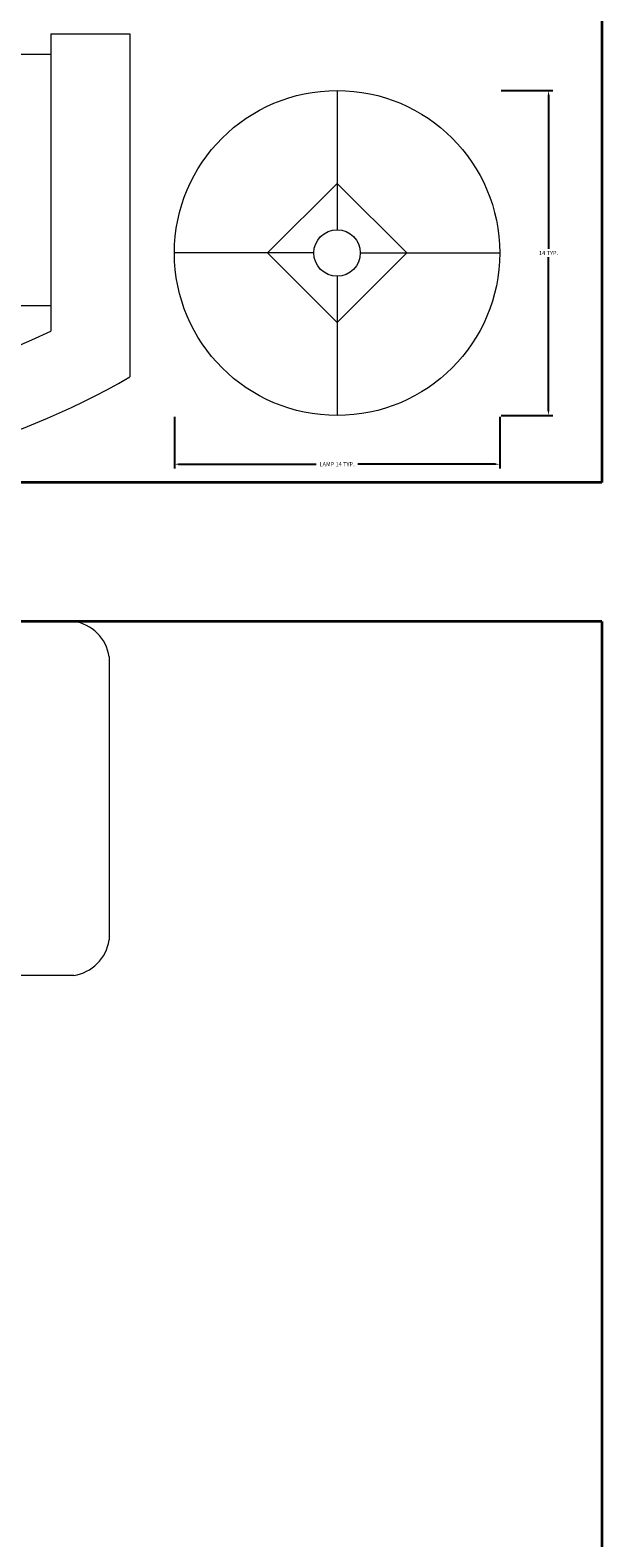
# Model space of a CAD drawing. Units: inches. Extents: x 4159 to 4826, y 299 to 1026.
# Tile 20 of 37: x 4423 to 4447, y 494 to 559. Entities that reach past the tile are written whole.
import ezdxf

# ---------------------------------------------------------------- set-up
doc = ezdxf.new("R2010")
doc.units = ezdxf.units.IN
for name, color, linetype, lineweight in [('A-ANNO-DIMS', 2, 'Continuous', 18), ('A-FURN', 8, 'Continuous', 18), ('A-WALL', 7, 'Continuous', 35)]:
    doc.layers.add(name, color=color, linetype=linetype, lineweight=lineweight)
doc.styles.get("Standard").update_dxf_attribs({"font": 'arial.ttf'})
doc.dimstyles.get("Standard").update_dxf_attribs({"dimtxt": 0.18, "dimasz": 0.18, "dimexe": 0.18, "dimexo": 0.0625, "dimgap": 0.09, "dimtad": 0, "dimtih": 1, "dimtoh": 1, "dimdec": 4, "dimzin": 0, "dimdsep": 46, "dimtxsty": 'Standard', "dimcen": 0.09, "dimadec": 0, "dimazin": 0, "dimtfac": 1, "dimtdec": 4, "dimtofl": 0, "dimtmove": 0, "dimatfit": 3, "dimfxl": 1, "dimtolj": 1, "dimtzin": 0, "dimarcsym": 0})

# ---------------------------------------------------------------- blocks, each defined once
blk = doc.blocks.new('Sofa - Roundback Loveseat 5 ft.')
for p, q in [((0, -32.44198), (0, -5.99998)), ((-24, -33.99998), (-24, -11.46958)), ((24.00004, -33.99998), (24.00004, -11.46958)), ((-23.9998, -13.38178), (23.99986, -13.38178)), ((-24, -32.44198), (24.00004, -32.44198))]:
    blk.add_line(p, q)
for points in [[(-24, -33.99998), (-30, -33.99998), (-30, -7.99998)], [(30.00004, -7.99998), (30.00004, -33.99998), (24.00004, -33.99998)]]:
    blk.add_lwpolyline(points)
for centre, radius, start, end in [((0, -60.24998), 60.24998, 60.13715, 119.8628), ((0, -61.38438), 55.38444, 64.32083, 115.6792)]:
    blk.add_arc(centre, radius, start, end)
blk = doc.blocks.new('Lamp - Table')
for p, q in [((0, 7), (0, 1)), ((0, 3), (-3, 0)), ((3, 0), (0, 3)), ((-1, 0), (-7, 0)), ((-3, 0), (0, -3)), ((0, -3), (3, 0)), ((1, 0), (7, 0)), ((0, -1), (0, -7))]:
    blk.add_line(p, q)
for radius in [7, 1]:
    blk.add_circle((0, 0), radius)
blk = doc.blocks.new('Desk - 30 x 60 in.')
for p, q in [((-26.999995, 0), (26.999995, 0)), ((-29.999995, -27), (-29.999995, -3)), ((29.999995, -3), (29.999995, -27)), ((26.999995, -30), (-26.999995, -30)), ((-20.000005, -30), (-20.000005, -31)), ((-16.000005, -31), (-16.000005, -30)), ((15.999995, -31), (15.999995, -30)), ((19.999995, -30), (19.999995, -31)), ((-20.000005, -31), (-16.000005, -31)), ((19.999995, -31), (15.999995, -31))]:
    blk.add_line(p, q)
for centre, start, end in [((-26.499995, -3.5), 98.1301, 171.8699), ((26.499995, -3.5), 8.130102, 81.8699), ((-26.499995, -26.5), 188.1301, 261.8699), ((26.499995, -26.5), 278.1301, 351.8699)]:
    blk.add_arc(centre, 3.535534, start, end)
blk = doc.blocks.new('*D33')
at = {"layer": 'A-ANNO-DIMS', "color": 0, "lineweight": -2, "transparency": 16777216}
for p, q in [((4428.862, 542.089), (4428.862, 539.865)), ((4442.904, 542.089), (4442.904, 539.865)), ((4429.042, 540.045), (4434.982, 540.045)), ((4442.724, 540.045), (4436.784, 540.045))]:
    blk.add_line(p, q, dxfattribs=at)
at = {"layer": 'A-ANNO-DIMS', "color": 0, "transparency": 16777216}
for points in [[(4429.042, 540.075), (4429.042, 540.015), (4428.862, 540.045)], [(4442.724, 540.075), (4442.724, 540.015), (4442.904, 540.045)]]:
    blk.add_solid(points, dxfattribs=at)
at = {"layer": 'Defpoints', "color": 0, "transparency": 16777216}
for p in [(4428.862, 542.152), (4442.904, 542.152), (4442.904, 540.045)]:
    blk.add_point(p, dxfattribs=at)
at = {"layer": 'A-ANNO-DIMS', "color": 0, "transparency": 16777216, "insert": (4435.883, 540.045), "char_height": 0.18, "attachment_point": 5}
blk.add_mtext('\\A1;LAMP 14 TYP.', dxfattribs=at)
blk = doc.blocks.new('*D34')
at = {"layer": 'A-ANNO-DIMS', "color": 0, "lineweight": -2, "transparency": 16777216}
for p, q in [((4442.967, 556.194), (4445.191, 556.194)), ((4445.011, 556.014), (4445.011, 549.353)), ((4445.011, 542.332), (4445.011, 548.993)), ((4442.967, 542.152), (4445.191, 542.152))]:
    blk.add_line(p, q, dxfattribs=at)
at = {"layer": 'A-ANNO-DIMS', "color": 0, "transparency": 16777216}
for points in [[(4444.981, 556.014), (4445.041, 556.014), (4445.011, 556.194)], [(4444.981, 542.332), (4445.041, 542.332), (4445.011, 542.152)]]:
    blk.add_solid(points, dxfattribs=at)
at = {"layer": 'Defpoints', "color": 0, "transparency": 16777216}
for p in [(4442.904, 556.194), (4445.011, 556.194), (4442.904, 542.152)]:
    blk.add_point(p, dxfattribs=at)
at = {"layer": 'A-ANNO-DIMS', "color": 0, "transparency": 16777216, "insert": (4445.011, 549.173), "char_height": 0.18, "attachment_point": 5}
blk.add_mtext('\\A1;14 TYP.', dxfattribs=at)
blk = doc.blocks.new('*D44')
at = {"layer": 'A-ANNO-DIMS', "color": 0, "lineweight": -2, "transparency": 16777216}
for p, q in [((4287.263, 963.093), (4158.88, 963.093)), ((4159.06, 962.913), (4159.06, 647.826)), ((4159.06, 332.375), (4159.06, 647.462)), ((4447.248, 332.195), (4158.88, 332.195))]:
    blk.add_line(p, q, dxfattribs=at)
at = {"layer": 'A-ANNO-DIMS', "color": 0, "transparency": 16777216}
for points in [[(4159.03, 962.913), (4159.09, 962.913), (4159.06, 963.093)], [(4159.03, 332.375), (4159.09, 332.375), (4159.06, 332.195)]]:
    blk.add_solid(points, dxfattribs=at)
at = {"layer": 'Defpoints', "color": 0, "transparency": 16777216}
for p in [(4287.326, 963.093), (4159.06, 332.195), (4447.31, 332.195)]:
    blk.add_point(p, dxfattribs=at)
at = {"layer": 'A-ANNO-DIMS', "color": 0, "transparency": 16777216, "insert": (4159.06, 647.644), "char_height": 0.18, "attachment_point": 5}
blk.add_mtext('\\A1;630.9', dxfattribs=at)

msp = doc.modelspace()

# ---------------------------------------------------------------- linework, layer by layer
at = {"layer": 'A-WALL'}
for p, q in [((4447.31, 618.254), (4447.31, 539.254)), ((4447.31, 539.254), (4369.31, 539.254)), ((4447.31, 533.254), (4369.31, 533.254)), ((4447.31, 533.254), (4447.31, 401.254))]:
    msp.add_line(p, q, dxfattribs=at)

# ---------------------------------------------------------------- block references
at = {"layer": 'A-FURN', "xscale": 0.5700533147329089, "yscale": 0.5700533147329089, "zscale": 0.5700533147329089, "rotation": 180}
msp.add_blockref('Sofa - Roundback Loveseat 5 ft.', (4409.841, 539.254), dxfattribs=at)
at = {"layer": 'A-FURN'}
for name, p, xscale, yscale, zscale in [('Lamp - Table', (4435.883, 549.173), 1.003057144141322, 1.003057144141322, 1.003057144141322), ('Desk - 30 x 60 in.', (4410.746, 533.254), 0.5098837128326598, 0.5098837128326598, 0.5098837128326598)]:
    msp.add_blockref(name, p, dxfattribs=dict(at, xscale=xscale, yscale=yscale, zscale=zscale))

# ---------------------------------------------------------------- dimensions: what is measured, and where the dimension line sits
at = {"layer": 'A-ANNO-DIMS'}
dim = msp.add_linear_dim(base=(4159.06, 332.195), p1=(4287.326, 963.093), p2=(4447.31, 332.195), angle=90, dimstyle='Standard', override={"dimdec": 1, "dimlfac": 1, "dimrnd": 0, "dimzin": 0, "dimdsep": 46, "dimlunit": 2}, dxfattribs=at)
dim.commit()
dim.dimension.update_dxf_attribs({"geometry": '*D44', "text_midpoint": (4159.06, 647.644)})
dim = msp.add_linear_dim(base=(4445.011, 556.194), p1=(4442.904, 542.152), p2=(4442.904, 556.194), angle=90, text='<> TYP.', dimstyle='Standard', override={"dimdec": 0, "dimlfac": 1, "dimrnd": 0, "dimzin": 0, "dimdsep": 46, "dimlunit": 2}, dxfattribs=at)
dim.commit()
dim.dimension.update_dxf_attribs({"geometry": '*D34', "text_midpoint": (4445.011, 549.173)})
dim = msp.add_linear_dim(base=(4442.904, 540.045), p1=(4428.862, 542.152), p2=(4442.904, 542.152), text='LAMP <> TYP.', dimstyle='Standard', override={"dimdec": 0, "dimlfac": 1, "dimrnd": 0, "dimzin": 0, "dimdsep": 46, "dimlunit": 2}, dxfattribs=at)
dim.commit()
dim.dimension.update_dxf_attribs({"geometry": '*D33', "text_midpoint": (4435.883, 540.045)})

doc.saveas('drawing.dxf')
